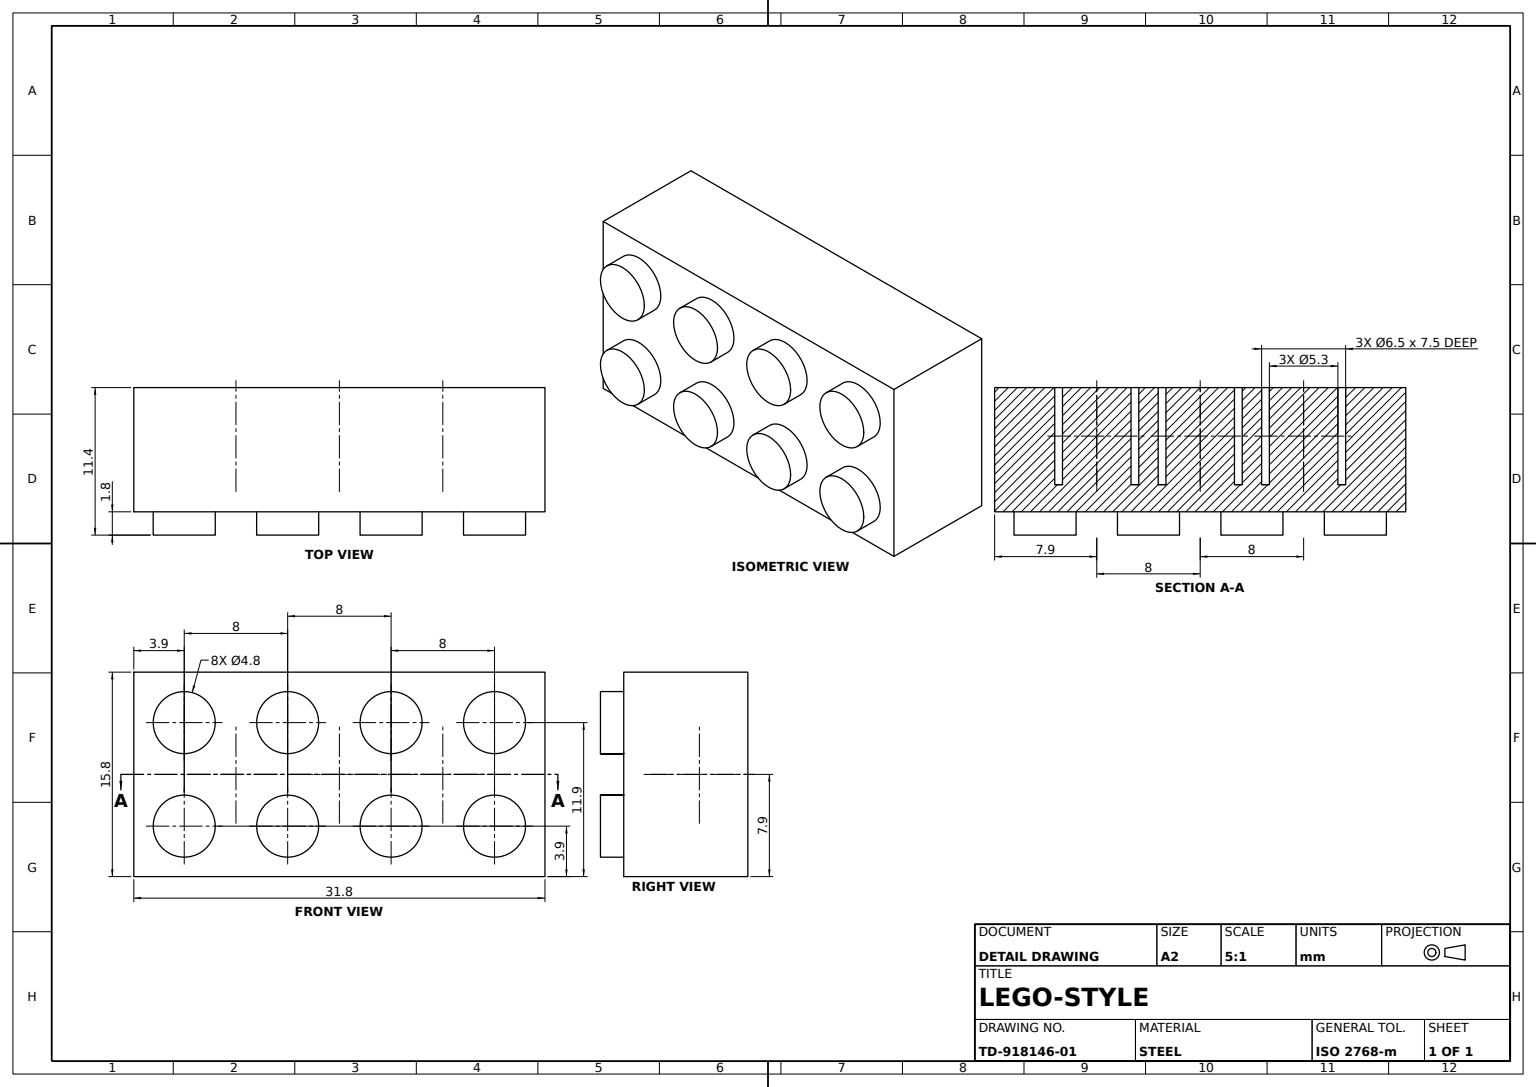
SolidWorks part; units mm, degrees
material "Plain Carbon Steel"
ref_plane "Front Plane" through (0, 0, 0) normal (0, 0, 1) x (1, 0, 0)
ref_plane "Top Plane" through (0, 0, 0) normal (0, 1, 0) x (1, 0, 0)
ref_plane "Right Plane" through (0, 0, 0) normal (1, 0, 0) x (0, 0, -1)
sketch "Brick Body Profile" plane through (0, 0, 0) normal (0, 0, 1) x (1, 0, 0)
  line L1 (-15.9, 7.9) -> (15.9, 7.9)
  line L2 (-15.9, 7.9) -> (-15.9, -7.9)
  line L3 (-15.9, -7.9) -> (15.9, -7.9)
  line L4 (15.9, 7.9) -> (15.9, -7.9)
  line L5 (-15.9, 7.9) -> (15.9, -7.9) construction
  line L6 (-15.9, -7.9) -> (15.9, 7.9) construction
  point P0 (0, 0)
  dimension "D1" = 31.8
  dimension "D2" = 15.8
extrude "Brick Body" add sketch "Brick Body Profile" along normal blind 9.6 contours L1 L4 L3 L2
sketch "Studs Profile 2x4 Ø4.8" plane through (0, 0, 9.6) normal (0, 0, 1) x (1, 0, 0)
  line L0 (-25.4971, 0) -> (37.7653, 0) construction
  line L1 (-15.9, 7.9) -> (-15.9, -7.9) construction
  circle A0 centre (-12, 4) radius 2.4
  circle A1 centre (-4, 4) radius 2.4
  circle A2 centre (4, 4) radius 2.4
  circle A3 centre (12, 4) radius 2.4
  circle A4 centre (12, -4) radius 2.4
  circle A5 centre (4, -4) radius 2.4
  circle A6 centre (-4, -4) radius 2.4
  circle A7 centre (-12, -4) radius 2.4
  dimension "D1" = 4.8
  dimension "D2" = 4
  dimension "D3" = 12
  dimension "D5" = 11.9
  dimension "D4" = 4
extrude "Studs 8xØ4.8" add sketch "Studs Profile 2x4 Ø4.8" along normal blind 1.8
sketch "Underside Cavity Profile" plane through (0, 0, 0) normal (0, 0, -1) x (-1, 0, 0)
  circle A0 centre (-8, 0) radius 3.25
  circle A1 centre (0, 0) radius 3.25
  circle A2 centre (8, 0) radius 3.25
  circle A3 centre (-8, 0) radius 2.65
  circle A4 centre (0, 0) radius 2.65
  circle A5 centre (8, 0) radius 2.65
  dimension "D1" = 6.5
  dimension "D4" = 5.3
  dimension "D2" = 8
  dimension "D3" = 8
extrude "Underside Cavity" cut sketch "Underside Cavity Profile" against normal blind 7.5 and the other way through all
